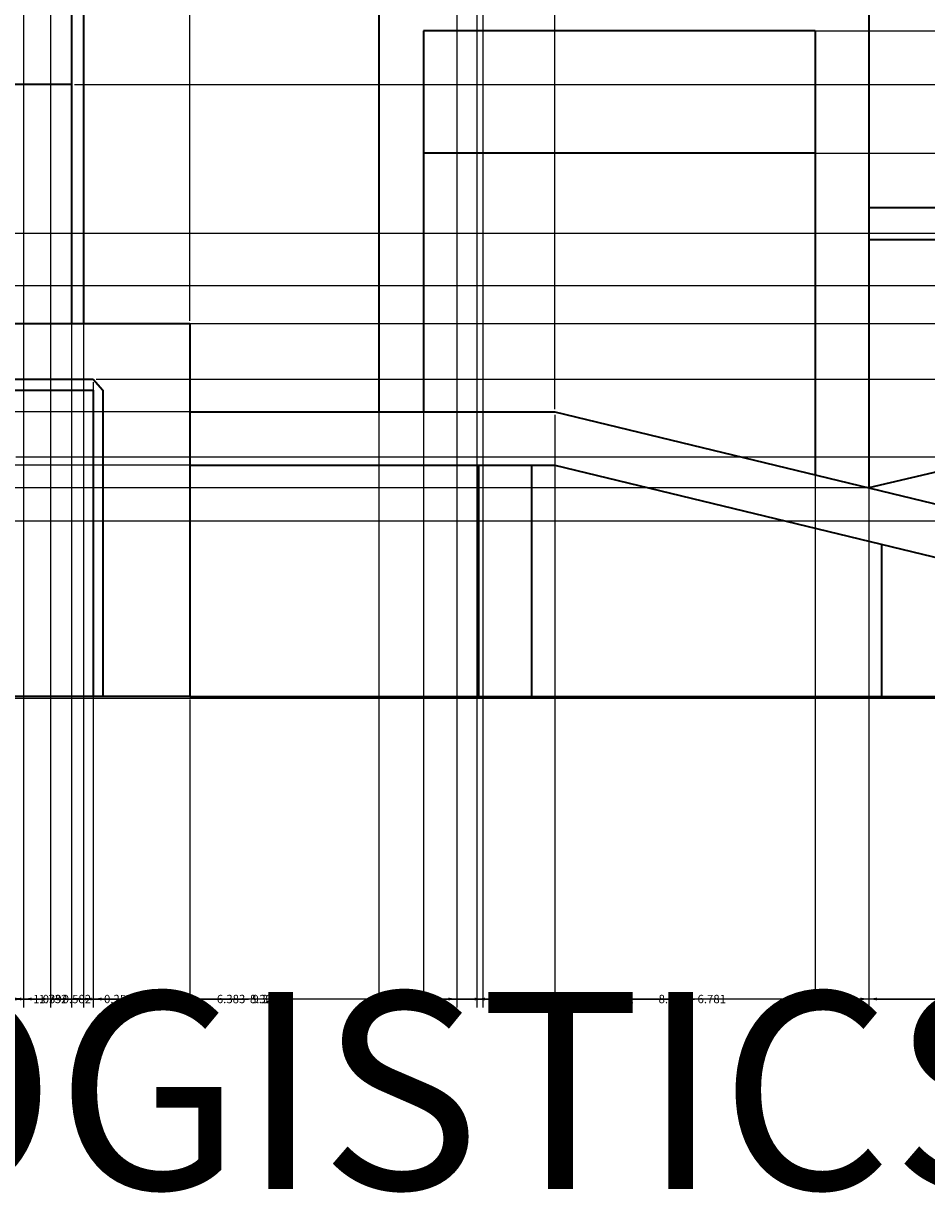
# Model space of a CAD drawing. Units: inches. Extents: x -10 to 130, y -32 to 34.
# Tile 14 of 22: x 71 to 90, y -32 to -7. Entities that reach past the tile are written whole.
import ezdxf

# ---------------------------------------------------------------- set-up
doc = ezdxf.new("R2010")
doc.units = ezdxf.units.IN
doc.header["$MEASUREMENT"] = 0
for name, color, linetype, lineweight in [('A-ANNO-DIMS', 2, 'Continuous', 18), ('A-ANNO-TEXT', 7, 'Continuous', 25), ('A-ELEV', 7, 'Continuous', 35)]:
    doc.layers.add(name, color=color, linetype=linetype, lineweight=lineweight)
doc.styles.get("Standard").update_dxf_attribs({"font": 'arial.ttf'})
doc.dimstyles.get("Standard").update_dxf_attribs({"dimtxt": 0.18, "dimasz": 0.18, "dimexe": 0.18, "dimexo": 0.0625, "dimgap": 0.09, "dimtad": 0, "dimtih": 1, "dimtoh": 1, "dimdec": 4, "dimzin": 0, "dimdsep": 46, "dimtxsty": 'Standard', "dimcen": 0.09, "dimadec": 0, "dimazin": 0, "dimtfac": 1, "dimtdec": 4, "dimtofl": 0, "dimtmove": 0, "dimatfit": 3, "dimfxl": 1, "dimtolj": 1, "dimtzin": 0, "dimarcsym": 0})

# ---------------------------------------------------------------- blocks, each defined once
blk = doc.blocks.new('*D1')
at = {"layer": 'A-ANNO-DIMS', "color": 0, "lineweight": -2, "transparency": 16777216}
for p, q in [((5.634, -13.647), (5.634, -28.129)), ((107.933, -21.477), (107.933, -28.129)), ((5.814, -27.949), (56.398, -27.949)), ((107.753, -27.949), (57.169, -27.949))]:
    blk.add_line(p, q, dxfattribs=at)
at = {"layer": 'A-ANNO-DIMS', "color": 0, "transparency": 16777216}
for points in [[(5.814, -27.919), (5.814, -27.979), (5.634, -27.949)], [(107.753, -27.919), (107.753, -27.979), (107.933, -27.949)]]:
    blk.add_solid(points, dxfattribs=at)
at = {"layer": 'Defpoints', "color": 0, "transparency": 16777216}
for p in [(5.634, -13.584), (107.933, -21.414), (107.933, -27.949)]:
    blk.add_point(p, dxfattribs=at)
at = {"layer": 'A-ANNO-DIMS', "color": 0, "transparency": 16777216, "insert": (56.784, -27.949), "char_height": 0.18, "attachment_point": 5}
blk.add_mtext('\\A1;102.3', dxfattribs=at)
blk = doc.blocks.new('*D2')
at = {"layer": 'A-ANNO-DIMS', "color": 0, "lineweight": -2, "transparency": 16777216}
for p, q in [((68.738, 27.199), (129.508, 27.199)), ((129.328, 27.019), (129.328, 3.074)), ((129.328, -21.234), (129.328, 2.71)), ((107.996, -21.414), (129.508, -21.414))]:
    blk.add_line(p, q, dxfattribs=at)
at = {"layer": 'A-ANNO-DIMS', "color": 0, "transparency": 16777216}
for points in [[(129.298, 27.019), (129.358, 27.019), (129.328, 27.199)], [(129.298, -21.234), (129.358, -21.234), (129.328, -21.414)]]:
    blk.add_solid(points, dxfattribs=at)
at = {"layer": 'Defpoints', "color": 0, "transparency": 16777216}
for p in [(68.676, 27.199), (129.328, 27.199), (107.933, -21.414)]:
    blk.add_point(p, dxfattribs=at)
at = {"layer": 'A-ANNO-DIMS', "color": 0, "transparency": 16777216, "insert": (129.328, 2.892), "char_height": 0.18, "attachment_point": 5}
blk.add_mtext('\\A1;48.61', dxfattribs=at)
blk = doc.blocks.new('*D47')
at = {"layer": 'A-ANNO-DIMS', "color": 0, "lineweight": -2, "transparency": 16777216}
for p, q in [((35.567, -12.534), (129.508, -12.534)), ((129.328, -12.714), (129.328, -16.792)), ((129.328, -21.234), (129.328, -17.156)), ((32.034, -21.414), (129.508, -21.414))]:
    blk.add_line(p, q, dxfattribs=at)
at = {"layer": 'A-ANNO-DIMS', "color": 0, "transparency": 16777216}
for points in [[(129.298, -12.714), (129.358, -12.714), (129.328, -12.534)], [(129.298, -21.234), (129.358, -21.234), (129.328, -21.414)]]:
    blk.add_solid(points, dxfattribs=at)
at = {"layer": 'Defpoints', "color": 0, "transparency": 16777216}
for p in [(35.505, -12.534), (31.971, -21.414), (129.328, -21.414)]:
    blk.add_point(p, dxfattribs=at)
at = {"layer": 'A-ANNO-DIMS', "color": 0, "transparency": 16777216, "insert": (129.328, -16.974), "char_height": 0.18, "attachment_point": 5}
blk.add_mtext('\\A1;8.88', dxfattribs=at)
blk = doc.blocks.new('*D48')
at = {"layer": 'A-ANNO-DIMS', "color": 0, "lineweight": -2, "transparency": 16777216}
for p, q in [((44.76, -13.293), (44.76, 33.879)), ((74.492, -13.293), (74.492, 33.879)), ((44.94, 33.699), (59.231, 33.699)), ((74.312, 33.699), (60.021, 33.699))]:
    blk.add_line(p, q, dxfattribs=at)
at = {"layer": 'A-ANNO-DIMS', "color": 0, "transparency": 16777216}
for points in [[(44.94, 33.729), (44.94, 33.669), (44.76, 33.699)], [(74.312, 33.729), (74.312, 33.669), (74.492, 33.699)]]:
    blk.add_solid(points, dxfattribs=at)
at = {"layer": 'Defpoints', "color": 0, "transparency": 16777216}
for p in [(74.492, 33.699), (44.76, -13.356), (74.492, -13.356)]:
    blk.add_point(p, dxfattribs=at)
at = {"layer": 'A-ANNO-DIMS', "color": 0, "transparency": 16777216, "insert": (59.626, 33.699), "char_height": 0.18, "attachment_point": 5}
blk.add_mtext('\\A1;29.73', dxfattribs=at)
blk = doc.blocks.new('*D55')
at = {"layer": 'A-ANNO-DIMS', "color": 0, "lineweight": -2, "transparency": 16777216}
for p, q in [((72.406, -14.617), (72.406, -28.129)), ((70.674, -16.297), (70.674, -28.129)), ((70.854, -27.949), (71.156, -27.949)), ((72.226, -27.949), (71.925, -27.949))]:
    blk.add_line(p, q, dxfattribs=at)
at = {"layer": 'A-ANNO-DIMS', "color": 0, "transparency": 16777216}
for points in [[(70.854, -27.919), (70.854, -27.979), (70.674, -27.949)], [(72.226, -27.919), (72.226, -27.979), (72.406, -27.949)]]:
    blk.add_solid(points, dxfattribs=at)
at = {"layer": 'Defpoints', "color": 0, "transparency": 16777216}
for p in [(72.406, -14.555), (70.674, -16.234), (72.406, -27.949)]:
    blk.add_point(p, dxfattribs=at)
at = {"layer": 'A-ANNO-DIMS', "color": 0, "transparency": 16777216, "insert": (71.54, -27.949), "char_height": 0.18, "attachment_point": 5}
blk.add_mtext('\\A1;1.732', dxfattribs=at)
blk = doc.blocks.new('*D56')
at = {"layer": 'A-ANNO-DIMS', "color": 0, "lineweight": -2, "transparency": 16777216}
for p, q in [((72.406, -14.617), (72.406, -28.129)), ((74.492, -21.477), (74.492, -28.129)), ((72.586, -27.949), (73.124, -27.949)), ((74.312, -27.949), (73.775, -27.949))]:
    blk.add_line(p, q, dxfattribs=at)
at = {"layer": 'A-ANNO-DIMS', "color": 0, "transparency": 16777216}
for points in [[(72.586, -27.919), (72.586, -27.979), (72.406, -27.949)], [(74.312, -27.919), (74.312, -27.979), (74.492, -27.949)]]:
    blk.add_solid(points, dxfattribs=at)
at = {"layer": 'Defpoints', "color": 0, "transparency": 16777216}
for p in [(72.406, -14.555), (74.492, -21.414), (74.492, -27.949)]:
    blk.add_point(p, dxfattribs=at)
at = {"layer": 'A-ANNO-DIMS', "color": 0, "transparency": 16777216, "insert": (73.449, -27.949), "char_height": 0.18, "attachment_point": 5}
blk.add_mtext('\\A1;2.09', dxfattribs=at)
blk = doc.blocks.new('*D57')
at = {"layer": 'A-ANNO-DIMS', "color": 0, "lineweight": -2, "transparency": 16777216}
for p, q in [((72.469, -14.555), (129.508, -14.555)), ((129.328, -14.735), (129.328, -17.803)), ((129.328, -21.234), (129.328, -18.167)), ((72.677, -21.414), (129.508, -21.414))]:
    blk.add_line(p, q, dxfattribs=at)
at = {"layer": 'A-ANNO-DIMS', "color": 0, "transparency": 16777216}
for points in [[(129.298, -14.735), (129.358, -14.735), (129.328, -14.555)], [(129.298, -21.234), (129.358, -21.234), (129.328, -21.414)]]:
    blk.add_solid(points, dxfattribs=at)
at = {"layer": 'Defpoints', "color": 0, "transparency": 16777216}
for p in [(72.406, -14.555), (72.614, -21.414), (129.328, -21.414)]:
    blk.add_point(p, dxfattribs=at)
at = {"layer": 'A-ANNO-DIMS', "color": 0, "transparency": 16777216, "insert": (129.328, -17.985), "char_height": 0.18, "attachment_point": 5}
blk.add_mtext('\\A1;6.86', dxfattribs=at)
blk = doc.blocks.new('*D58')
at = {"layer": 'A-ANNO-DIMS', "color": 0, "lineweight": -2, "transparency": 16777216}
for p, q in [((70.737, -16.234), (129.508, -16.234)), ((129.328, -16.414), (129.328, -18.66)), ((129.328, -21.269), (129.328, -19.024)), ((70.737, -21.449), (129.508, -21.449))]:
    blk.add_line(p, q, dxfattribs=at)
at = {"layer": 'A-ANNO-DIMS', "color": 0, "transparency": 16777216}
for points in [[(129.298, -16.414), (129.358, -16.414), (129.328, -16.234)], [(129.298, -21.269), (129.358, -21.269), (129.328, -21.449)]]:
    blk.add_solid(points, dxfattribs=at)
at = {"layer": 'Defpoints', "color": 0, "transparency": 16777216}
for p in [(70.674, -16.234), (70.674, -21.449), (129.328, -21.449)]:
    blk.add_point(p, dxfattribs=at)
at = {"layer": 'A-ANNO-DIMS', "color": 0, "transparency": 16777216, "insert": (129.328, -18.842), "char_height": 0.18, "attachment_point": 5}
blk.add_mtext('\\A1;5.215', dxfattribs=at)
blk = doc.blocks.new('*D59')
at = {"layer": 'A-ANNO-DIMS', "color": 0, "lineweight": -2, "transparency": 16777216}
for p, q in [((64.975, -17.615), (129.508, -17.615)), ((129.328, -17.795), (129.328, -19.35)), ((129.328, -21.269), (129.328, -19.714)), ((64.975, -21.449), (129.508, -21.449))]:
    blk.add_line(p, q, dxfattribs=at)
at = {"layer": 'A-ANNO-DIMS', "color": 0, "transparency": 16777216}
for points in [[(129.298, -17.795), (129.358, -17.795), (129.328, -17.615)], [(129.298, -21.269), (129.358, -21.269), (129.328, -21.449)]]:
    blk.add_solid(points, dxfattribs=at)
at = {"layer": 'Defpoints', "color": 0, "transparency": 16777216}
for p in [(64.913, -17.615), (64.913, -21.449), (129.328, -21.449)]:
    blk.add_point(p, dxfattribs=at)
at = {"layer": 'A-ANNO-DIMS', "color": 0, "transparency": 16777216, "insert": (129.328, -19.532), "char_height": 0.18, "attachment_point": 5}
blk.add_mtext('\\A1;3.835', dxfattribs=at)
blk = doc.blocks.new('*D60')
at = {"layer": 'A-ANNO-DIMS', "color": 0, "lineweight": -2, "transparency": 16777216}
for p, q in [((74.492, -13.293), (74.492, 33.879)), ((82.377, -15.202), (82.377, 33.879)), ((74.672, 33.699), (78.041, 33.699)), ((82.197, 33.699), (78.828, 33.699))]:
    blk.add_line(p, q, dxfattribs=at)
at = {"layer": 'A-ANNO-DIMS', "color": 0, "transparency": 16777216}
for points in [[(74.672, 33.729), (74.672, 33.669), (74.492, 33.699)], [(82.197, 33.729), (82.197, 33.669), (82.377, 33.699)]]:
    blk.add_solid(points, dxfattribs=at)
at = {"layer": 'Defpoints', "color": 0, "transparency": 16777216}
for p in [(82.377, 33.699), (74.492, -13.356), (82.377, -15.264)]:
    blk.add_point(p, dxfattribs=at)
at = {"layer": 'A-ANNO-DIMS', "color": 0, "transparency": 16777216, "insert": (78.435, 33.699), "char_height": 0.18, "attachment_point": 5}
blk.add_mtext('\\A1;7.885', dxfattribs=at)
blk = doc.blocks.new('*D61')
at = {"layer": 'A-ANNO-DIMS', "color": 0, "lineweight": -2, "transparency": 16777216}
for p, q in [((82.377, -15.327), (82.377, -28.129)), ((89.158, -21.477), (89.158, -28.129)), ((82.557, -27.949), (85.391, -27.949)), ((88.978, -27.949), (86.144, -27.949))]:
    blk.add_line(p, q, dxfattribs=at)
at = {"layer": 'A-ANNO-DIMS', "color": 0, "transparency": 16777216}
for points in [[(82.557, -27.919), (82.557, -27.979), (82.377, -27.949)], [(88.978, -27.919), (88.978, -27.979), (89.158, -27.949)]]:
    blk.add_solid(points, dxfattribs=at)
at = {"layer": 'Defpoints', "color": 0, "transparency": 16777216}
for p in [(82.377, -15.264), (89.158, -21.414), (89.158, -27.949)]:
    blk.add_point(p, dxfattribs=at)
at = {"layer": 'A-ANNO-DIMS', "color": 0, "transparency": 16777216, "insert": (85.767, -27.949), "char_height": 0.18, "attachment_point": 5}
blk.add_mtext('\\A1;6.781', dxfattribs=at)
blk = doc.blocks.new('*D62')
at = {"layer": 'A-ANNO-DIMS', "color": 0, "lineweight": -2, "transparency": 16777216}
for p, q in [((89.158, -21.477), (89.158, -28.129)), ((103.018, -21.477), (103.018, -28.129)), ((89.338, -27.949), (95.703, -27.949)), ((102.838, -27.949), (96.473, -27.949))]:
    blk.add_line(p, q, dxfattribs=at)
at = {"layer": 'A-ANNO-DIMS', "color": 0, "transparency": 16777216}
for points in [[(89.338, -27.919), (89.338, -27.979), (89.158, -27.949)], [(102.838, -27.919), (102.838, -27.979), (103.018, -27.949)]]:
    blk.add_solid(points, dxfattribs=at)
at = {"layer": 'Defpoints', "color": 0, "transparency": 16777216}
for p in [(89.158, -21.414), (103.018, -21.414), (103.018, -27.949)]:
    blk.add_point(p, dxfattribs=at)
at = {"layer": 'A-ANNO-DIMS', "color": 0, "transparency": 16777216, "insert": (96.088, -27.949), "char_height": 0.18, "attachment_point": 5}
blk.add_mtext('\\A1;13.86', dxfattribs=at)
blk = doc.blocks.new('*D64')
at = {"layer": 'A-ANNO-DIMS', "color": 0, "lineweight": -2, "transparency": 16777216}
for p, q in [((82.315, -15.264), (-9.564, -15.264)), ((-9.384, -15.444), (-9.384, -15.659)), ((-9.384, -16.237), (-9.384, -16.022)), ((82.315, -16.417), (-9.564, -16.417))]:
    blk.add_line(p, q, dxfattribs=at)
at = {"layer": 'A-ANNO-DIMS', "color": 0, "transparency": 16777216}
for points in [[(-9.414, -15.444), (-9.354, -15.444), (-9.384, -15.264)], [(-9.414, -16.237), (-9.354, -16.237), (-9.384, -16.417)]]:
    blk.add_solid(points, dxfattribs=at)
at = {"layer": 'Defpoints', "color": 0, "transparency": 16777216}
for p in [(82.377, -15.264), (-9.384, -16.417), (82.377, -16.417)]:
    blk.add_point(p, dxfattribs=at)
at = {"layer": 'A-ANNO-DIMS', "color": 0, "transparency": 16777216, "insert": (-9.384, -15.841), "char_height": 0.18, "attachment_point": 5}
blk.add_mtext('\\A1;1.15', dxfattribs=at)
blk = doc.blocks.new('*D65')
at = {"layer": 'A-ANNO-DIMS', "color": 0, "lineweight": -2, "transparency": 16777216}
for p, q in [((82.315, -16.417), (-9.564, -16.417)), ((-9.384, -16.597), (-9.384, -18.734)), ((-9.384, -21.234), (-9.384, -19.097)), ((80.669, -21.414), (-9.564, -21.414))]:
    blk.add_line(p, q, dxfattribs=at)
at = {"layer": 'A-ANNO-DIMS', "color": 0, "transparency": 16777216}
for points in [[(-9.414, -16.597), (-9.354, -16.597), (-9.384, -16.417)], [(-9.414, -21.234), (-9.354, -21.234), (-9.384, -21.414)]]:
    blk.add_solid(points, dxfattribs=at)
at = {"layer": 'Defpoints', "color": 0, "transparency": 16777216}
for p in [(-9.384, -16.417), (82.377, -16.417), (80.731, -21.414)]:
    blk.add_point(p, dxfattribs=at)
at = {"layer": 'A-ANNO-DIMS', "color": 0, "transparency": 16777216, "insert": (-9.384, -18.916), "char_height": 0.18, "attachment_point": 5}
blk.add_mtext('\\A1;4.998', dxfattribs=at)
blk = doc.blocks.new('*D66')
at = {"layer": 'A-ANNO-DIMS', "color": 0, "lineweight": -2, "transparency": 16777216}
for p, q in [((89.158, -16.844), (89.158, 33.879)), ((104.453, -13.219), (104.453, 33.879)), ((89.338, 33.699), (96.35, 33.699)), ((104.273, 33.699), (97.261, 33.699))]:
    blk.add_line(p, q, dxfattribs=at)
at = {"layer": 'A-ANNO-DIMS', "color": 0, "transparency": 16777216}
for points in [[(89.338, 33.729), (89.338, 33.669), (89.158, 33.699)], [(104.273, 33.729), (104.273, 33.669), (104.453, 33.699)]]:
    blk.add_solid(points, dxfattribs=at)
at = {"layer": 'Defpoints', "color": 0, "transparency": 16777216}
for p in [(104.453, 33.699), (104.453, -13.282), (89.158, -16.906)]:
    blk.add_point(p, dxfattribs=at)
at = {"layer": 'A-ANNO-DIMS', "color": 0, "transparency": 16777216, "insert": (96.805, 33.699), "char_height": 0.18, "attachment_point": 5}
blk.add_mtext('\\A1;15.295', dxfattribs=at)
blk = doc.blocks.new('*D69')
at = {"layer": 'A-ANNO-DIMS', "color": 0, "lineweight": -2, "transparency": 16777216}
for p, q in [((89.095, -16.906), (-9.564, -16.906)), ((-9.384, -17.086), (-9.384, -18.979)), ((-9.384, -21.234), (-9.384, -19.342)), ((89.095, -21.414), (-9.564, -21.414))]:
    blk.add_line(p, q, dxfattribs=at)
at = {"layer": 'A-ANNO-DIMS', "color": 0, "transparency": 16777216}
for points in [[(-9.414, -17.086), (-9.354, -17.086), (-9.384, -16.906)], [(-9.414, -21.234), (-9.354, -21.234), (-9.384, -21.414)]]:
    blk.add_solid(points, dxfattribs=at)
at = {"layer": 'Defpoints', "color": 0, "transparency": 16777216}
for p in [(89.158, -16.906), (-9.384, -21.414), (89.158, -21.414)]:
    blk.add_point(p, dxfattribs=at)
at = {"layer": 'A-ANNO-DIMS', "color": 0, "transparency": 16777216, "insert": (-9.384, -19.16), "char_height": 0.18, "attachment_point": 5}
blk.add_mtext('\\A1;4.508', dxfattribs=at)
blk = doc.blocks.new('*D75')
at = {"layer": 'A-ANNO-DIMS', "color": 0, "lineweight": -2, "transparency": 16777216}
for p, q in [((62.588, -11.398), (129.508, -11.398)), ((129.328, -11.578), (129.328, -12.195)), ((129.328, -13.176), (129.328, -12.559)), ((62.588, -13.356), (129.508, -13.356))]:
    blk.add_line(p, q, dxfattribs=at)
at = {"layer": 'A-ANNO-DIMS', "color": 0, "transparency": 16777216}
for points in [[(129.298, -11.578), (129.358, -11.578), (129.328, -11.398)], [(129.298, -13.176), (129.358, -13.176), (129.328, -13.356)]]:
    blk.add_solid(points, dxfattribs=at)
at = {"layer": 'Defpoints', "color": 0, "transparency": 16777216}
for p in [(62.526, -11.398), (129.328, -11.398), (62.526, -13.356)]:
    blk.add_point(p, dxfattribs=at)
at = {"layer": 'A-ANNO-DIMS', "color": 0, "transparency": 16777216, "insert": (129.328, -12.377), "char_height": 0.18, "attachment_point": 5}
blk.add_mtext('\\A1;1.96', dxfattribs=at)
blk = doc.blocks.new('*D76')
at = {"layer": 'A-ANNO-DIMS', "color": 0, "lineweight": -2, "transparency": 16777216}
for p, q in [((62.588, -6.485), (129.508, -6.485)), ((129.328, -6.665), (129.328, -8.76)), ((129.328, -11.218), (129.328, -9.123)), ((62.588, -11.398), (129.508, -11.398))]:
    blk.add_line(p, q, dxfattribs=at)
at = {"layer": 'A-ANNO-DIMS', "color": 0, "transparency": 16777216}
for points in [[(129.298, -6.665), (129.358, -6.665), (129.328, -6.485)], [(129.298, -11.218), (129.358, -11.218), (129.328, -11.398)]]:
    blk.add_solid(points, dxfattribs=at)
at = {"layer": 'Defpoints', "color": 0, "transparency": 16777216}
for p in [(62.526, -6.485), (129.328, -6.485), (62.526, -11.398)]:
    blk.add_point(p, dxfattribs=at)
at = {"layer": 'A-ANNO-DIMS', "color": 0, "transparency": 16777216, "insert": (129.328, -8.942), "char_height": 0.18, "attachment_point": 5}
blk.add_mtext('\\A1;4.913', dxfattribs=at)
blk = doc.blocks.new('*D151')
at = {"layer": 'A-ANNO-DIMS', "color": 0, "lineweight": -2, "transparency": 16777216}
for p, q in [((71.48, 1.942), (71.48, -28.129)), ((70.898, 1.448), (70.898, -28.129)), ((71.078, -27.949), (71.3, -27.949)), ((71.48, -27.949), (71.66, -27.949))]:
    blk.add_line(p, q, dxfattribs=at)
at = {"layer": 'A-ANNO-DIMS', "color": 0, "transparency": 16777216}
for points in [[(71.078, -27.919), (71.078, -27.979), (70.898, -27.949)], [(71.3, -27.919), (71.3, -27.979), (71.48, -27.949)]]:
    blk.add_solid(points, dxfattribs=at)
at = {"layer": 'Defpoints', "color": 0, "transparency": 16777216}
for p in [(71.48, 2.005), (70.898, 1.511), (71.48, -27.949)]:
    blk.add_point(p, dxfattribs=at)
at = {"layer": 'A-ANNO-DIMS', "color": 0, "transparency": 16777216, "insert": (72.053, -27.949), "char_height": 0.18, "attachment_point": 5}
blk.add_mtext('\\A1;0.582', dxfattribs=at)
blk = doc.blocks.new('*D152')
at = {"layer": 'A-ANNO-DIMS', "color": 0, "lineweight": -2, "transparency": 16777216}
for p, q in [((71.48, 1.942), (71.48, -28.129)), ((80.823, 1.942), (80.823, -28.129)), ((71.66, -27.949), (75.758, -27.949)), ((80.643, -27.949), (76.545, -27.949))]:
    blk.add_line(p, q, dxfattribs=at)
at = {"layer": 'A-ANNO-DIMS', "color": 0, "transparency": 16777216}
for points in [[(71.66, -27.919), (71.66, -27.979), (71.48, -27.949)], [(80.643, -27.919), (80.643, -27.979), (80.823, -27.949)]]:
    blk.add_solid(points, dxfattribs=at)
at = {"layer": 'Defpoints', "color": 0, "transparency": 16777216}
for p in [(71.48, 2.005), (80.823, 2.005), (80.823, -27.949)]:
    blk.add_point(p, dxfattribs=at)
at = {"layer": 'A-ANNO-DIMS', "color": 0, "transparency": 16777216, "insert": (76.152, -27.949), "char_height": 0.18, "attachment_point": 5}
blk.add_mtext('\\A1;9.343', dxfattribs=at)
blk = doc.blocks.new('*D155')
at = {"layer": 'A-ANNO-DIMS', "color": 0, "lineweight": -2, "transparency": 16777216}
for p, q in [((70.897993, 1.448166), (70.897993, -28.129305)), ((71.936707, 1.448166), (71.936707, -28.129305)), ((70.717993, -27.949305), (70.537993, -27.949305)), ((72.116707, -27.949305), (72.296707, -27.949305))]:
    blk.add_line(p, q, dxfattribs=at)
at = {"layer": 'A-ANNO-DIMS', "color": 0, "transparency": 16777216}
for points in [[(70.717993, -27.919305), (70.717993, -27.979305), (70.897993, -27.949305)], [(72.116707, -27.919305), (72.116707, -27.979305), (71.936707, -27.949305)]]:
    blk.add_solid(points, dxfattribs=at)
at = {"layer": 'Defpoints', "color": 0, "transparency": 16777216}
for p in [(70.897993, 1.510666), (71.936707, 1.510666), (71.936707, -27.949305)]:
    blk.add_point(p, dxfattribs=at)
at = {"layer": 'A-ANNO-DIMS', "color": 0, "transparency": 16777216, "insert": (71.41735, -27.949305), "char_height": 0.18, "attachment_point": 5}
blk.add_mtext('\\A1;1.039', dxfattribs=at)
blk = doc.blocks.new('*D156')
at = {"layer": 'A-ANNO-DIMS', "color": 0, "lineweight": -2, "transparency": 16777216}
for p, q in [((71.937, -6.284), (71.937, -28.129)), ((80.26, -6.284), (80.26, -28.129)), ((72.117, -27.949), (75.704, -27.949)), ((80.08, -27.949), (76.492, -27.949))]:
    blk.add_line(p, q, dxfattribs=at)
at = {"layer": 'A-ANNO-DIMS', "color": 0, "transparency": 16777216}
for points in [[(72.117, -27.919), (72.117, -27.979), (71.937, -27.949)], [(80.08, -27.919), (80.08, -27.979), (80.26, -27.949)]]:
    blk.add_solid(points, dxfattribs=at)
at = {"layer": 'Defpoints', "color": 0, "transparency": 16777216}
for p in [(71.937, -6.222), (80.26, -6.222), (80.26, -27.949)]:
    blk.add_point(p, dxfattribs=at)
at = {"layer": 'A-ANNO-DIMS', "color": 0, "transparency": 16777216, "insert": (76.098, -27.949), "char_height": 0.18, "attachment_point": 5}
blk.add_mtext('\\A1;8.323', dxfattribs=at)
blk = doc.blocks.new('*D157')
at = {"layer": 'A-ANNO-DIMS', "color": 0, "lineweight": -2, "transparency": 16777216}
for p, q in [((80.26, -6.284), (80.26, -28.129)), ((80.691, -6.284), (80.691, -28.129)), ((80.08, -27.949), (79.9, -27.949)), ((80.871, -27.949), (81.051, -27.949))]:
    blk.add_line(p, q, dxfattribs=at)
at = {"layer": 'A-ANNO-DIMS', "color": 0, "transparency": 16777216}
for points in [[(80.08, -27.919), (80.08, -27.979), (80.26, -27.949)], [(80.871, -27.919), (80.871, -27.979), (80.691, -27.949)]]:
    blk.add_solid(points, dxfattribs=at)
at = {"layer": 'Defpoints', "color": 0, "transparency": 16777216}
for p in [(80.26, -6.222), (80.691, -6.222), (80.691, -27.949)]:
    blk.add_point(p, dxfattribs=at)
at = {"layer": 'A-ANNO-DIMS', "color": 0, "transparency": 16777216, "insert": (81.444, -27.949), "char_height": 0.18, "attachment_point": 5}
blk.add_mtext('\\A1;0.432', dxfattribs=at)
blk = doc.blocks.new('*D158')
at = {"layer": 'A-ANNO-DIMS', "color": 0, "lineweight": -2, "transparency": 16777216}
for p, q in [((80.691, -6.284), (80.691, -28.129)), ((89.158, -6.284), (89.158, -28.129)), ((80.871, -27.949), (84.531, -27.949)), ((88.978, -27.949), (85.318, -27.949))]:
    blk.add_line(p, q, dxfattribs=at)
at = {"layer": 'A-ANNO-DIMS', "color": 0, "transparency": 16777216}
for points in [[(80.871, -27.919), (80.871, -27.979), (80.691, -27.949)], [(88.978, -27.919), (88.978, -27.979), (89.158, -27.949)]]:
    blk.add_solid(points, dxfattribs=at)
at = {"layer": 'Defpoints', "color": 0, "transparency": 16777216}
for p in [(80.691, -6.222), (89.158, -6.222), (89.158, -27.949)]:
    blk.add_point(p, dxfattribs=at)
at = {"layer": 'A-ANNO-DIMS', "color": 0, "transparency": 16777216, "insert": (84.925, -27.949), "char_height": 0.18, "attachment_point": 5}
blk.add_mtext('\\A1;8.466', dxfattribs=at)
blk = doc.blocks.new('*D159')
at = {"layer": 'A-ANNO-DIMS', "color": 0, "lineweight": -2, "transparency": 16777216}
for p, q in [((89.158, -6.284), (89.158, -28.129)), ((94.73, -6.284), (94.73, -28.129)), ((89.338, -27.949), (91.551, -27.949)), ((94.55, -27.949), (92.337, -27.949))]:
    blk.add_line(p, q, dxfattribs=at)
at = {"layer": 'A-ANNO-DIMS', "color": 0, "transparency": 16777216}
for points in [[(89.338, -27.919), (89.338, -27.979), (89.158, -27.949)], [(94.55, -27.919), (94.55, -27.979), (94.73, -27.949)]]:
    blk.add_solid(points, dxfattribs=at)
at = {"layer": 'Defpoints', "color": 0, "transparency": 16777216}
for p in [(89.158, -6.222), (94.73, -6.222), (94.73, -27.949)]:
    blk.add_point(p, dxfattribs=at)
at = {"layer": 'A-ANNO-DIMS', "color": 0, "transparency": 16777216, "insert": (91.944, -27.949), "char_height": 0.18, "attachment_point": 5}
blk.add_mtext('\\A1;5.572', dxfattribs=at)
blk = doc.blocks.new('*D167')
at = {"layer": 'A-ANNO-DIMS', "color": 0, "lineweight": -2, "transparency": 16777216}
for p, q in [((71.937, -13.418), (71.937, -28.129)), ((72.193, -13.418), (72.193, -28.129)), ((71.757, -27.949), (71.577, -27.949)), ((72.373, -27.949), (72.553, -27.949))]:
    blk.add_line(p, q, dxfattribs=at)
at = {"layer": 'A-ANNO-DIMS', "color": 0, "transparency": 16777216}
for points in [[(71.757, -27.919), (71.757, -27.979), (71.937, -27.949)], [(72.373, -27.919), (72.373, -27.979), (72.193, -27.949)]]:
    blk.add_solid(points, dxfattribs=at)
at = {"layer": 'Defpoints', "color": 0, "transparency": 16777216}
for p in [(71.937, -13.356), (72.193, -13.356), (72.193, -27.949)]:
    blk.add_point(p, dxfattribs=at)
at = {"layer": 'A-ANNO-DIMS', "color": 0, "transparency": 16777216, "insert": (72.946, -27.949), "char_height": 0.18, "attachment_point": 5}
blk.add_mtext('\\A1;0.256', dxfattribs=at)
blk = doc.blocks.new('*D168')
at = {"layer": 'A-ANNO-DIMS', "color": 0, "lineweight": -2, "transparency": 16777216}
for p, q in [((71.999, -6.222), (129.508, -6.222)), ((129.328, -6.402), (129.328, -7.024)), ((129.328, -8.009), (129.328, -7.387)), ((71.999, -8.189), (129.508, -8.189))]:
    blk.add_line(p, q, dxfattribs=at)
at = {"layer": 'A-ANNO-DIMS', "color": 0, "transparency": 16777216}
for points in [[(129.298, -6.402), (129.358, -6.402), (129.328, -6.222)], [(129.298, -8.009), (129.358, -8.009), (129.328, -8.189)]]:
    blk.add_solid(points, dxfattribs=at)
at = {"layer": 'Defpoints', "color": 0, "transparency": 16777216}
for p in [(71.937, -6.222), (71.937, -8.189), (129.328, -8.189)]:
    blk.add_point(p, dxfattribs=at)
at = {"layer": 'A-ANNO-DIMS', "color": 0, "transparency": 16777216, "insert": (129.328, -7.205), "char_height": 0.18, "attachment_point": 5}
blk.add_mtext('\\A1;1.967', dxfattribs=at)
blk = doc.blocks.new('*D169')
at = {"layer": 'A-ANNO-DIMS', "color": 0, "lineweight": -2, "transparency": 16777216}
for p, q in [((72.193, -6.284), (72.193, -28.129)), ((78.576, -6.284), (78.576, -28.129)), ((72.373, -27.949), (74.99, -27.949)), ((78.396, -27.949), (75.779, -27.949))]:
    blk.add_line(p, q, dxfattribs=at)
at = {"layer": 'A-ANNO-DIMS', "color": 0, "transparency": 16777216}
for points in [[(72.373, -27.919), (72.373, -27.979), (72.193, -27.949)], [(78.396, -27.919), (78.396, -27.979), (78.576, -27.949)]]:
    blk.add_solid(points, dxfattribs=at)
at = {"layer": 'Defpoints', "color": 0, "transparency": 16777216}
for p in [(72.193, -6.222), (78.576, -6.222), (78.576, -27.949)]:
    blk.add_point(p, dxfattribs=at)
at = {"layer": 'A-ANNO-DIMS', "color": 0, "transparency": 16777216, "insert": (75.384, -27.949), "char_height": 0.18, "attachment_point": 5}
blk.add_mtext('\\A1;6.383', dxfattribs=at)
blk = doc.blocks.new('*D170')
at = {"layer": 'A-ANNO-DIMS', "color": 0, "lineweight": -2, "transparency": 16777216}
for p, q in [((79.539, -7.093), (79.539, -28.129)), ((88.002, -7.093), (88.002, -28.129)), ((79.719, -27.949), (83.378, -27.949)), ((87.822, -27.949), (84.163, -27.949))]:
    blk.add_line(p, q, dxfattribs=at)
at = {"layer": 'A-ANNO-DIMS', "color": 0, "transparency": 16777216}
for points in [[(79.719, -27.919), (79.719, -27.979), (79.539, -27.949)], [(87.822, -27.919), (87.822, -27.979), (88.002, -27.949)]]:
    blk.add_solid(points, dxfattribs=at)
at = {"layer": 'Defpoints', "color": 0, "transparency": 16777216}
for p in [(79.539, -7.03), (88.002, -7.03), (88.002, -27.949)]:
    blk.add_point(p, dxfattribs=at)
at = {"layer": 'A-ANNO-DIMS', "color": 0, "transparency": 16777216, "insert": (83.771, -27.949), "char_height": 0.18, "attachment_point": 5}
blk.add_mtext('\\A1;8.462', dxfattribs=at)
blk = doc.blocks.new('*D171')
at = {"layer": 'A-ANNO-DIMS', "color": 0, "lineweight": -2, "transparency": 16777216}
for p, q in [((79.602, -7.03), (129.508, -7.03)), ((129.328, -7.21), (129.328, -8.167)), ((129.328, -9.489), (129.328, -8.531)), ((79.602, -9.669), (129.508, -9.669))]:
    blk.add_line(p, q, dxfattribs=at)
at = {"layer": 'A-ANNO-DIMS', "color": 0, "transparency": 16777216}
for points in [[(129.298, -7.21), (129.358, -7.21), (129.328, -7.03)], [(129.298, -9.489), (129.358, -9.489), (129.328, -9.669)]]:
    blk.add_solid(points, dxfattribs=at)
at = {"layer": 'Defpoints', "color": 0, "transparency": 16777216}
for p in [(79.539, -7.03), (79.539, -9.669), (129.328, -9.669)]:
    blk.add_point(p, dxfattribs=at)
at = {"layer": 'A-ANNO-DIMS', "color": 0, "transparency": 16777216, "insert": (129.328, -8.349), "char_height": 0.18, "attachment_point": 5}
blk.add_mtext('\\A1;2.639', dxfattribs=at)
blk = doc.blocks.new('*D172')
at = {"layer": 'A-ANNO-DIMS', "color": 0, "lineweight": -2, "transparency": 16777216}
for p, q in [((89.22, -6.222), (129.508, -6.222)), ((129.328, -6.402), (129.328, -6.85)), ((88.064, -7.03), (129.508, -7.03)), ((129.328, -7.03), (129.328, -7.21)), ((129.328, -7.21), (129.148, -7.21))]:
    blk.add_line(p, q, dxfattribs=at)
at = {"layer": 'A-ANNO-DIMS', "color": 0, "transparency": 16777216}
for points in [[(129.298, -6.402), (129.358, -6.402), (129.328, -6.222)], [(129.298, -6.85), (129.358, -6.85), (129.328, -7.03)]]:
    blk.add_solid(points, dxfattribs=at)
at = {"layer": 'Defpoints', "color": 0, "transparency": 16777216}
for p in [(89.158, -6.222), (88.002, -7.03), (129.328, -7.03)]:
    blk.add_point(p, dxfattribs=at)
at = {"layer": 'A-ANNO-DIMS', "color": 0, "transparency": 16777216, "insert": (128.754, -7.21), "char_height": 0.18, "attachment_point": 5}
blk.add_mtext('\\A1;0.808', dxfattribs=at)
blk = doc.blocks.new('*D173')
at = {"layer": 'A-ANNO-DIMS', "color": 0, "lineweight": -2, "transparency": 16777216}
for p, q in [((89.158, -10.906), (89.158, -28.129)), ((99.96, -10.906), (99.96, -28.129)), ((89.338, -27.949), (94.105, -27.949)), ((99.78, -27.949), (95.013, -27.949))]:
    blk.add_line(p, q, dxfattribs=at)
at = {"layer": 'A-ANNO-DIMS', "color": 0, "transparency": 16777216}
for points in [[(89.338, -27.919), (89.338, -27.979), (89.158, -27.949)], [(99.78, -27.919), (99.78, -27.979), (99.96, -27.949)]]:
    blk.add_solid(points, dxfattribs=at)
at = {"layer": 'Defpoints', "color": 0, "transparency": 16777216}
for p in [(89.158, -10.843), (99.96, -10.843), (99.96, -27.949)]:
    blk.add_point(p, dxfattribs=at)
at = {"layer": 'A-ANNO-DIMS', "color": 0, "transparency": 16777216, "insert": (94.559, -27.949), "char_height": 0.18, "attachment_point": 5}
blk.add_mtext('\\A1;10.802', dxfattribs=at)

msp = doc.modelspace()

# ---------------------------------------------------------------- linework, layer by layer
at = {"layer": 'A-ELEV'}
for p, q in [((71.9367, -6.2218), (71.9367, -13.3558)), ((72.1928, -6.2218), (72.1928, -13.3558)), ((78.5759, -6.2218), (78.5759, -15.2645)), ((89.1578, -6.2218), (89.1578, -16.1883)), ((79.5394, -7.0301), (79.5394, -15.2645)), ((88.0017, -7.0301), (79.5394, -7.0301)), ((88.0017, -7.0301), (88.0017, -16.6264)), ((71.9367, -8.1891), (64.8443, -8.1891)), ((88.0017, -9.6688), (79.5394, -9.6688)), ((89.1578, -10.8435), (107.9333, -10.8435)), ((89.1578, -11.5395), (107.2998, -11.5395)), ((64.8443, -13.3558), (74.492, -13.3558)), ((74.492, -13.3558), (74.492, -21.4145)), ((104.4531, -13.2819), (89.1578, -16.9063)), ((64.8443, -14.555), (72.4063, -14.555)), ((72.4063, -14.555), (72.6144, -14.7925)), ((64.8443, -14.7925), (72.4063, -14.7925)), ((72.4063, -14.7925), (72.4063, -21.4145)), ((72.6144, -14.7925), (72.6144, -21.4145)), ((74.492, -15.2645), (82.377, -15.2645)), ((82.377, -15.2645), (107.7767, -21.4145)), ((74.492, -16.4166), (82.377, -16.4166)), ((80.7314, -16.4166), (80.7314, -21.4145)), ((81.8739, -16.4166), (81.8739, -21.4145)), ((82.377, -16.4166), (103.0183, -21.4145)), ((89.1578, -16.1883), (89.1578, -16.9063)), ((89.4315, -18.1247), (89.4315, -21.4145)), ((74.492, -21.4145), (64.913, -21.4145)), ((74.492, -21.4145), (89.1578, -21.4145)), ((89.1578, -21.4145), (99.9603, -21.4145))]:
    msp.add_line(p, q, dxfattribs=at)

# ---------------------------------------------------------------- texts
at = {"layer": 'A-ANNO-TEXT'}
msp.add_text('REAR   ELEVATION    AND   LOGISTICS   HUB', height=4.256275, dxfattribs=at).set_placement((-5.4651, -32.0569))

# ---------------------------------------------------------------- dimensions: what is measured, and where the dimension line sits
at = {"layer": 'A-ANNO-DIMS'}
for base, p1, p2, override, picture, middle in [((74.492, 33.6987), (44.76, -13.3558), (74.492, -13.3558), {"dimdec": 2, "dimlfac": 1, "dimrnd": 0, "dimzin": 0, "dimdsep": 46, "dimlunit": 2}, '*D48', (59.626, 33.6987)), ((82.377, 33.6987), (74.492, -13.3558), (82.377, -15.2645), {"dimdec": 3, "dimlfac": 1, "dimrnd": 0, "dimzin": 0, "dimdsep": 46, "dimlunit": 2}, '*D60', (78.4345, 33.6987)), ((104.4531, 33.6987), (89.1578, -16.9063), (104.4531, -13.2819), {"dimdec": 3, "dimlfac": 1, "dimrnd": 0, "dimzin": 0, "dimdsep": 46, "dimlunit": 2}, '*D66', (96.8055, 33.6987)), ((71.4801, -27.9493), (70.898, 1.5107), (71.4801, 2.0049), {"dimdec": 3, "dimlfac": 1, "dimrnd": 0, "dimzin": 0, "dimdsep": 46, "dimlunit": 2}, '*D151', (72.0529, -27.9493)), ((80.8232, -27.9493), (71.4801, 2.0049), (80.8232, 2.0049), {"dimdec": 3, "dimlfac": 1, "dimrnd": 0, "dimzin": 0, "dimdsep": 46, "dimlunit": 2}, '*D152', (76.1517, -27.9493)), ((71.9367, -27.9493), (70.898, 1.5107), (71.9367, 1.5107), {"dimdec": 3, "dimlfac": 1, "dimrnd": 0, "dimzin": 0, "dimdsep": 46, "dimlunit": 2}, '*D155', (71.4173, -27.9493)), ((80.2599, -27.9493), (71.9367, -6.2218), (80.2599, -6.2218), {"dimdec": 3, "dimlfac": 1, "dimrnd": 0, "dimzin": 0, "dimdsep": 46, "dimlunit": 2}, '*D156', (76.0983, -27.9493)), ((78.5759, -27.9493), (72.1928, -6.2218), (78.5759, -6.2218), {"dimdec": 3, "dimlfac": 1, "dimrnd": 0, "dimzin": 0, "dimdsep": 46, "dimlunit": 2}, '*D169', (75.3844, -27.9493)), ((80.69143, -27.9493), (80.25986, -6.22179), (80.69143, -6.22179), {"dimdec": 3, "dimlfac": 1, "dimrnd": 0, "dimzin": 0, "dimdsep": 46, "dimlunit": 2}, '*D157', (81.44421, -27.9493)), ((89.1578, -27.9493), (80.6914, -6.2218), (89.1578, -6.2218), {"dimdec": 3, "dimlfac": 1, "dimrnd": 0, "dimzin": 0, "dimdsep": 46, "dimlunit": 2}, '*D158', (84.9246, -27.9493)), ((94.7302, -27.9493), (89.1578, -6.2218), (94.7302, -6.2218), {"dimdec": 3, "dimlfac": 1, "dimrnd": 0, "dimzin": 0, "dimdsep": 46, "dimlunit": 2}, '*D159', (91.944, -27.9493)), ((88.0017, -27.9493), (79.5394, -7.0301), (88.0017, -7.0301), {"dimdec": 3, "dimlfac": 1, "dimrnd": 0, "dimzin": 0, "dimdsep": 46, "dimlunit": 2}, '*D170', (83.7705, -27.9493)), ((99.96027, -27.9493), (89.15784, -10.84347), (99.96027, -10.84347), {"dimdec": 3, "dimlfac": 1, "dimrnd": 0, "dimzin": 0, "dimdsep": 46, "dimlunit": 2}, '*D173', (94.55905, -27.9493)), ((72.1928, -27.9493), (71.9367, -13.3558), (72.1928, -13.3558), {"dimdec": 3, "dimlfac": 1, "dimrnd": 0, "dimzin": 0, "dimdsep": 46, "dimlunit": 2}, '*D167', (72.9464, -27.9493)), ((107.9333, -27.9493), (5.634, -13.5841), (107.9333, -21.4145), {"dimdec": 1, "dimlfac": 1, "dimrnd": 0, "dimzin": 0, "dimdsep": 46, "dimlunit": 2}, '*D1', (56.7837, -27.9493)), ((72.4063, -27.9493), (70.6743, -16.2341), (72.4063, -14.555), {"dimdec": 3, "dimlfac": 1, "dimrnd": 0, "dimzin": 0, "dimdsep": 46, "dimlunit": 2}, '*D55', (71.5403, -27.9493)), ((74.492, -27.9493), (72.4063, -14.555), (74.492, -21.4145), {"dimdec": 2, "dimlfac": 1, "dimrnd": 0, "dimzin": 0, "dimdsep": 46, "dimlunit": 2}, '*D56', (73.4492, -27.9493)), ((89.1578, -27.9493), (82.377, -15.2645), (89.1578, -21.4145), {"dimdec": 3, "dimlfac": 1, "dimrnd": 0, "dimzin": 0, "dimdsep": 46, "dimlunit": 2}, '*D61', (85.7674, -27.9493)), ((103.0183, -27.9493), (89.1578, -21.4145), (103.0183, -21.4145), {"dimdec": 2, "dimlfac": 1, "dimrnd": 0, "dimzin": 0, "dimdsep": 46, "dimlunit": 2}, '*D62', (96.0881, -27.9493))]:
    dim = msp.add_linear_dim(base=base, p1=p1, p2=p2, dimstyle='Standard', override=override, dxfattribs=at)
    dim.commit()
    dim.dimension.update_dxf_attribs({"geometry": picture, "text_midpoint": middle})
for base, p1, p2, override, picture, middle in [((129.3277, 27.1987), (107.9333, -21.4145), (68.6759, 27.1987), {"dimdec": 2, "dimlfac": 1, "dimrnd": 0, "dimzin": 0, "dimdsep": 46, "dimlunit": 2}, '*D2', (129.3277, 2.8921)), ((129.3277, -8.1891), (71.9367, -6.2218), (71.9367, -8.1891), {"dimdec": 3, "dimlfac": 1, "dimrnd": 0, "dimzin": 0, "dimdsep": 46, "dimlunit": 2}, '*D168', (129.3277, -7.2054)), ((129.3277, -7.0301), (89.1578, -6.2218), (88.0017, -7.0301), {"dimdec": 3, "dimlfac": 1, "dimrnd": 0, "dimzin": 0, "dimdsep": 46, "dimlunit": 2}, '*D172', (128.7538, -7.2101)), ((129.3277, -6.4849), (62.5256, -11.3982), (62.5256, -6.4849), {"dimdec": 3, "dimlfac": 1, "dimrnd": 0, "dimzin": 0, "dimdsep": 46, "dimlunit": 2}, '*D76', (129.3277, -8.9415)), ((129.3277, -9.6688), (79.5394, -7.0301), (79.5394, -9.6688), {"dimdec": 3, "dimlfac": 1, "dimrnd": 0, "dimzin": 0, "dimdsep": 46, "dimlunit": 2}, '*D171', (129.3277, -8.3494)), ((129.3277, -11.3982), (62.5256, -13.3558), (62.5256, -11.3982), {"dimdec": 2, "dimlfac": 1, "dimrnd": 0, "dimzin": 0, "dimdsep": 46, "dimlunit": 2}, '*D75', (129.3277, -12.377)), ((129.3277, -21.4145), (35.5046, -12.5339), (31.9712, -21.4145), {"dimdec": 2, "dimlfac": 1, "dimrnd": 0, "dimzin": 0, "dimdsep": 46, "dimlunit": 2}, '*D47', (129.3277, -16.9742)), ((129.3277, -21.4145), (72.4063, -14.555), (72.6144, -21.4145), {"dimdec": 2, "dimlfac": 1, "dimrnd": 0, "dimzin": 0, "dimdsep": 46, "dimlunit": 2}, '*D57', (129.3277, -17.9847)), ((-9.3836, -16.4166), (82.377, -15.2645), (82.377, -16.4166), {"dimdec": 2, "dimlfac": 1, "dimrnd": 0, "dimzin": 0, "dimdsep": 46, "dimlunit": 2}, '*D64', (-9.3836, -15.8406)), ((-9.3836, -16.4166), (80.7314, -21.4145), (82.377, -16.4166), {"dimdec": 3, "dimlfac": 1, "dimrnd": 0, "dimzin": 0, "dimdsep": 46, "dimlunit": 2}, '*D65', (-9.3836, -18.9156)), ((129.3277, -21.4493), (70.6743, -16.2341), (70.6743, -21.4493), {"dimdec": 3, "dimlfac": 1, "dimrnd": 0, "dimzin": 0, "dimdsep": 46, "dimlunit": 2}, '*D58', (129.3277, -18.8417)), ((-9.3836, -21.4145), (89.1578, -16.9063), (89.1578, -21.4145), {"dimdec": 3, "dimlfac": 1, "dimrnd": 0, "dimzin": 0, "dimdsep": 46, "dimlunit": 2}, '*D69', (-9.3836, -19.1604)), ((129.3277, -21.4493), (64.913, -17.6146), (64.913, -21.4493), {"dimdec": 3, "dimlfac": 1, "dimrnd": 0, "dimzin": 0, "dimdsep": 46, "dimlunit": 2}, '*D59', (129.3277, -19.532))]:
    dim = msp.add_linear_dim(base=base, p1=p1, p2=p2, angle=90, dimstyle='Standard', override=override, dxfattribs=at)
    dim.commit()
    dim.dimension.update_dxf_attribs({"geometry": picture, "text_midpoint": middle})

doc.saveas('drawing.dxf')
